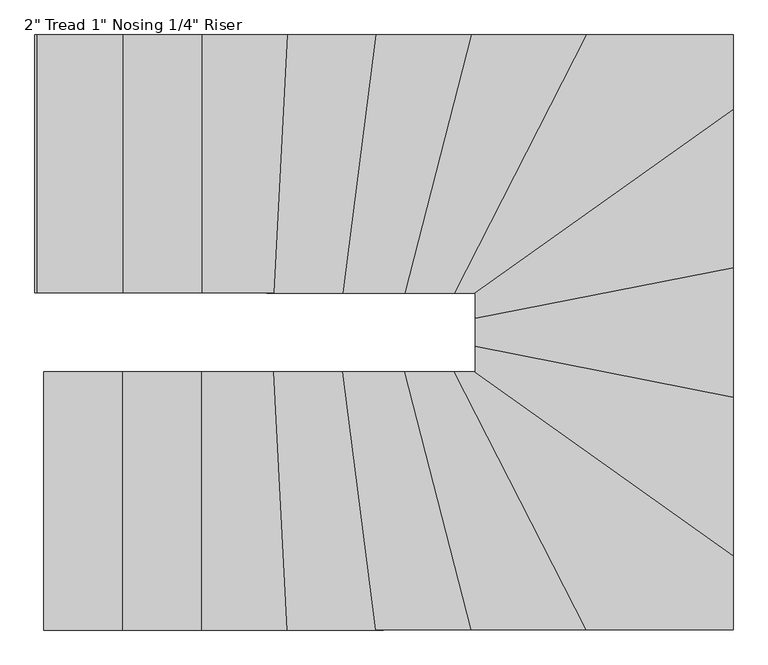
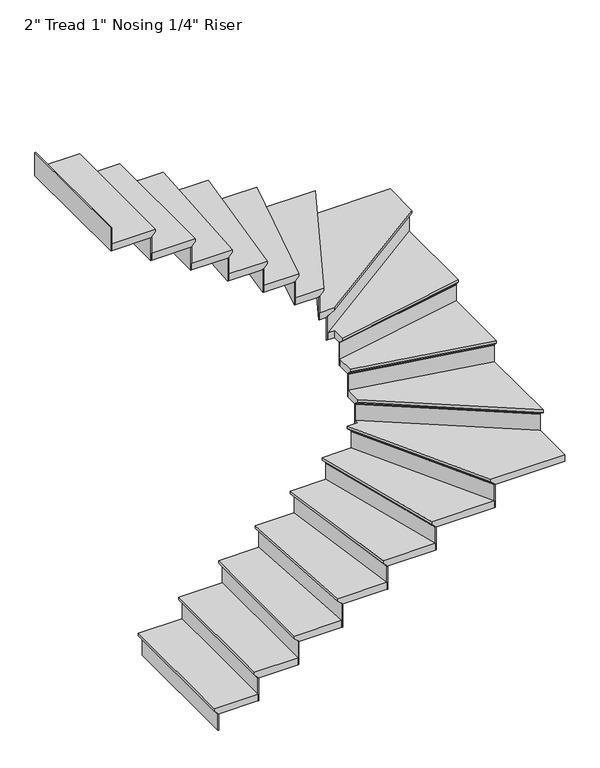
"""IFC4 building model written with IfcOpenShell, lengths in millimetres: stair flight geometry."""

from ifc_helpers import new_model, si_unit, origin, place, context, project, spatial, faceted_brep, source, transform, mapped, element, save


def stair_flight_4f848c3a(model_context):
    return source(origin(), model_context, "Body", "Brep", [
        faceted_brep([(531.7538115, -7565.2090409, 3350.6833333), (531.7538115, -7565.2090409, 3369.7333333), (531.7538115, -6650.8090409, 3369.7333333), (531.7538115, -6650.8090409, 3350.6833333), (557.1538115, -7565.2090409, 3325.2833333), (557.1538115, -6650.8090409, 3325.2833333), (836.5538115, -7565.2090409, 3369.7333333), (836.5538115, -6650.8090409, 3369.7333333), (557.1538115, -6650.8090409, 3318.9333333), (836.5538115, -6650.8090409, 3318.9333333), (836.5538115, -7565.2090409, 3318.9333333), (557.1538115, -7565.2090409, 3318.9333333)], [[[0, 1, 2, 3]], [[4, 0, 3, 5]], [[2, 1, 6, 7]], [[8, 9, 10, 11]], [[2, 7, 9, 8, 5, 3]], [[8, 11, 4, 5]], [[6, 1, 0, 4, 11, 10]], [[7, 6, 10, 9]]]),
        faceted_brep([(557.1538115, -7565.2090409, 3318.9333333), (557.1538115, -7565.2090409, 3200.4), (563.5038115, -7565.2090409, 3200.4), (563.5038115, -7565.2090409, 3318.9333333), (557.1538115, -6650.8090409, 3318.9333333), (563.5038115, -6650.8090409, 3318.9333333), (563.5038115, -6650.8090409, 3200.4), (557.1538115, -6650.8090409, 3200.4)], [[[0, 1, 2, 3]], [[4, 5, 6, 7]], [[1, 0, 4, 7]], [[2, 1, 7, 6]], [[3, 2, 6, 5]], [[0, 3, 5, 4]]]),
        faceted_brep([(836.5538115, -7565.2090409, 3488.2666667), (836.5538115, -7565.2090409, 3318.9333333), (842.9038115, -7565.2090409, 3318.9333333), (842.9038115, -7565.2090409, 3488.2666667), (836.5538115, -6650.8090409, 3488.2666667), (842.9038115, -6650.8090409, 3488.2666667), (842.9038115, -6650.8090409, 3318.9333333), (836.5538115, -6650.8090409, 3318.9333333)], [[[0, 1, 2, 3]], [[4, 5, 6, 7]], [[1, 0, 4, 7]], [[2, 1, 7, 6]], [[3, 2, 6, 5]], [[0, 3, 5, 4]]]),
        faceted_brep([(811.1538115, -6650.8090409, 3539.0666667), (811.1538115, -7565.2090409, 3539.0666667), (1115.9538115, -7565.2090409, 3539.0666667), (1115.9538115, -6650.8090409, 3539.0666667), (836.5538115, -6650.8090409, 3488.2666667), (1115.9538115, -6650.8090409, 3488.2666667), (1115.9538115, -7565.2090409, 3488.2666667), (836.5538115, -7565.2090409, 3488.2666667), (836.5538115, -6650.8090409, 3494.6166667), (811.1538115, -6650.8090409, 3520.0166667), (836.5538115, -7565.2090409, 3494.6166667), (811.1538115, -7565.2090409, 3520.0166667)], [[[0, 1, 2, 3]], [[4, 5, 6, 7]], [[0, 3, 5, 4, 8, 9]], [[4, 7, 10, 8]], [[2, 1, 11, 10, 7, 6]], [[3, 2, 6, 5]], [[11, 1, 0, 9]], [[10, 11, 9, 8]]]),
        faceted_brep([(1115.9538115, -7565.2090409, 3657.6), (1115.9538115, -7565.2090409, 3488.2666667), (1122.3038115, -7565.2090409, 3488.2666667), (1122.3038115, -7565.2090409, 3657.6), (1115.9538115, -6650.8090409, 3657.6), (1122.3038115, -6650.8090409, 3657.6), (1122.3038115, -6650.8090409, 3488.2666667), (1115.9538115, -6650.8090409, 3488.2666667)], [[[0, 1, 2, 3]], [[4, 5, 6, 7]], [[1, 0, 4, 7]], [[2, 1, 7, 6]], [[3, 2, 6, 5]], [[0, 3, 5, 4]]]),
        faceted_brep([(1090.5538115, -6650.8090409, 3708.4), (1090.5538115, -7565.2090409, 3708.4), (1419.1552434, -7565.2090409, 3708.4), (1371.620973, -6650.8090409, 3708.4), (1115.9538115, -6650.8090409, 3657.6), (1371.620973, -6650.8090409, 3657.6), (1419.1552434, -7565.2090409, 3657.6), (1115.9538115, -7565.2090409, 3657.6), (1115.9538115, -6650.8090409, 3663.95), (1090.5538115, -6650.8090409, 3689.35), (1115.9538115, -7565.2090409, 3663.95), (1090.5538115, -7565.2090409, 3689.35)], [[[0, 1, 2, 3]], [[4, 5, 6, 7]], [[0, 3, 5, 4, 8, 9]], [[4, 7, 10, 8]], [[2, 1, 11, 10, 7, 6]], [[3, 2, 6, 5]], [[11, 1, 0, 9]], [[10, 11, 9, 8]]]),
        faceted_brep([(1419.1552434, -7565.2090409, 3826.9333333), (1419.1552434, -7565.2090409, 3657.6), (1425.5138176, -7565.2090409, 3657.6), (1425.5138176, -7565.2090409, 3826.9333333), (1371.620973, -6650.8090409, 3826.9333333), (1377.9795471, -6650.8090409, 3826.9333333), (1377.9795471, -6650.8090409, 3657.6), (1371.620973, -6650.8090409, 3657.6)], [[[0, 1, 2, 3]], [[4, 5, 6, 7]], [[1, 0, 4, 7]], [[2, 1, 7, 6]], [[3, 2, 6, 5]], [[0, 3, 5, 4]]]),
        faceted_brep([(1346.1866763, -6650.8090409, 3877.7333333), (1393.7209467, -7565.2090409, 3877.7333333), (1734.1437245, -7565.2090409, 3877.7333333), (1615.7876728, -6650.8090409, 3877.7333333), (1371.620973, -6650.8090409, 3826.9333333), (1615.7876728, -6650.8090409, 3826.9333333), (1734.1437245, -7565.2090409, 3826.9333333), (1419.1552434, -7565.2090409, 3826.9333333), (1371.620973, -6650.8090409, 3833.2833333), (1346.1866763, -6650.8090409, 3858.6833333), (1419.1552434, -7565.2090409, 3833.2833333), (1393.7209467, -7565.2090409, 3858.6833333)], [[[0, 1, 2, 3]], [[4, 5, 6, 7]], [[0, 3, 5, 4, 8, 9]], [[4, 7, 10, 8]], [[2, 1, 11, 10, 7, 6]], [[3, 2, 6, 5]], [[11, 1, 0, 9]], [[10, 11, 9, 8]]]),
        faceted_brep([(1734.1437245, -7565.2090409, 3996.2666667), (1734.1437245, -7565.2090409, 3826.9333333), (1740.5466962, -7565.2090409, 3826.9333333), (1740.5466962, -7565.2090409, 3996.2666667), (1615.7876728, -6650.8090409, 3996.2666667), (1622.1906446, -6650.8090409, 3996.2666667), (1622.1906446, -6650.8090409, 3826.9333333), (1615.7876728, -6650.8090409, 3826.9333333)], [[[0, 1, 2, 3]], [[4, 5, 6, 7]], [[1, 0, 4, 7]], [[2, 1, 7, 6]], [[3, 2, 6, 5]], [[0, 3, 5, 4]]]),
        faceted_brep([(1590.1757857, -6650.8090409, 4047.0666667), (1708.5318374, -7565.2090409, 4047.0666667), (2072.5453427, -7565.2090409, 4047.0666667), (1837.4148953, -6650.8090409, 4047.0666667), (1615.7876728, -6650.8090409, 3996.2666667), (1837.4148953, -6650.8090409, 3996.2666667), (2072.5453427, -7565.2090409, 3996.2666667), (1734.1437245, -7565.2090409, 3996.2666667), (1615.7876728, -6650.8090409, 4002.6166667), (1590.1757857, -6650.8090409, 4028.0166667), (1734.1437245, -7565.2090409, 4002.6166667), (1708.5318374, -7565.2090409, 4028.0166667)], [[[0, 1, 2, 3]], [[4, 5, 6, 7]], [[0, 3, 5, 4, 8, 9]], [[4, 7, 10, 8]], [[2, 1, 11, 10, 7, 6]], [[3, 2, 6, 5]], [[11, 1, 0, 9]], [[10, 11, 9, 8]]]),
        faceted_brep([(2072.5453427, -7565.2090409, 4165.6), (2072.5453427, -7565.2090409, 3996.2666667), (2079.1019196, -7565.2090409, 3996.2666667), (2079.1019196, -7565.2090409, 4165.6), (1837.4148953, -6650.8090409, 4165.6), (1843.9714722, -6650.8090409, 4165.6), (1843.9714722, -6650.8090409, 3996.2666667), (1837.4148953, -6650.8090409, 3996.2666667)], [[[0, 1, 2, 3]], [[4, 5, 6, 7]], [[1, 0, 4, 7]], [[2, 1, 7, 6]], [[3, 2, 6, 5]], [[0, 3, 5, 4]]]),
        faceted_brep([(1811.1885878, -6650.8090409, 4216.4), (2046.3190352, -7565.2090409, 4216.4), (2482.5861527, -7565.2090409, 4216.4), (2013.7615314, -6650.8090409, 4216.4), (1837.4148953, -6650.8090409, 4165.6), (2013.7615314, -6650.8090409, 4165.6), (2482.5861527, -7565.2090409, 4165.6), (2072.5453427, -7565.2090409, 4165.6), (1837.4148953, -6650.8090409, 4171.95), (1811.1885878, -6650.8090409, 4197.35), (2072.5453427, -7565.2090409, 4171.95), (2046.3190352, -7565.2090409, 4197.35)], [[[0, 1, 2, 3]], [[4, 5, 6, 7]], [[0, 3, 5, 4, 8, 9]], [[4, 7, 10, 8]], [[2, 1, 11, 10, 7, 6]], [[3, 2, 6, 5]], [[11, 1, 0, 9]], [[10, 11, 9, 8]]]),
        faceted_brep([(2482.5861527, -7565.2090409, 4334.9333333), (2482.5861527, -7565.2090409, 4165.6), (2489.7221358, -7565.2090409, 4165.6), (2489.7221358, -7565.2090409, 4334.9333333), (2013.7615314, -6650.8090409, 4334.9333333), (2020.8975145, -6650.8090409, 4334.9333333), (2020.8975145, -6650.8090409, 4165.6), (2013.7615314, -6650.8090409, 4165.6)], [[[0, 1, 2, 3]], [[4, 5, 6, 7]], [[1, 0, 4, 7]], [[2, 1, 7, 6]], [[3, 2, 6, 5]], [[0, 3, 5, 4]]]),
        faceted_brep([(2059.4855034, -6621.253958, 4385.7333333), (2059.4855034, -6650.8090409, 4385.7333333), (1985.2175988, -6650.8090409, 4385.7333333), (2454.0422202, -7565.2090409, 4385.7333333), (2973.8855034, -7565.2090409, 4385.7333333), (2973.8855034, -7271.5279072, 4385.7333333), (2059.4855034, -6650.8090409, 4334.9333333), (2059.4855034, -6621.253958, 4334.9333333), (2973.8855034, -7271.5279072, 4334.9333333), (2973.8855034, -7565.2090409, 4334.9333333), (2482.5861527, -7565.2090409, 4334.9333333), (2013.7615314, -6650.8090409, 4334.9333333), (2013.7615314, -6650.8090409, 4341.2833333), (1985.2175988, -6650.8090409, 4366.6833333), (2482.5861527, -7565.2090409, 4341.2833333), (2454.0422202, -7565.2090409, 4366.6833333)], [[[0, 1, 2, 3, 4, 5]], [[6, 7, 8, 9, 10, 11]], [[1, 0, 7, 6]], [[2, 1, 6, 11, 12, 13]], [[11, 10, 14, 12]], [[4, 3, 15, 14, 10, 9]], [[5, 4, 9, 8]], [[0, 5, 8, 7]], [[15, 3, 2, 13]], [[14, 15, 13, 12]]]),
        faceted_brep([(2973.8855034, -7271.5279072, 4504.2666667), (2973.8855034, -7271.5279072, 4334.9333333), (2973.8855034, -7263.7359324, 4334.9333333), (2973.8855034, -7263.7359324, 4504.2666667), (2059.4855034, -6621.253958, 4504.2666667), (2059.4855034, -6613.4619832, 4504.2666667), (2059.4855034, -6613.4619832, 4334.9333333), (2059.4855034, -6621.253958, 4334.9333333)], [[[0, 1, 2, 3]], [[4, 5, 6, 7]], [[1, 0, 4, 7]], [[2, 1, 7, 6]], [[3, 2, 6, 5]], [[0, 3, 5, 4]]]),
        faceted_brep([(2059.4855034, -6652.4218572, 4555.0666667), (2973.8855034, -7302.6958063, 4555.0666667), (2973.8855034, -6715.0407273, 4555.0666667), (2059.4855034, -6534.7998709, 4555.0666667), (2059.4855034, -6621.253958, 4504.2666667), (2059.4855034, -6534.7998709, 4504.2666667), (2973.8855034, -6715.0407273, 4504.2666667), (2973.8855034, -7271.5279072, 4504.2666667), (2059.4855034, -6621.253958, 4510.6166667), (2059.4855034, -6652.4218572, 4536.0166667), (2973.8855034, -7271.5279072, 4510.6166667), (2973.8855034, -7302.6958063, 4536.0166667)], [[[0, 1, 2, 3]], [[4, 5, 6, 7]], [[0, 3, 5, 4, 8, 9]], [[4, 7, 10, 8]], [[3, 2, 6, 5]], [[11, 1, 0, 9]], [[10, 11, 9, 8]], [[2, 1, 11, 10, 7, 6]]]),
        faceted_brep([(2973.8855034, -6715.0407273, 4673.6), (2973.8855034, -6715.0407273, 4504.2666667), (2973.8855034, -6708.5685418, 4504.2666667), (2973.8855034, -6708.5685418, 4673.6), (2059.4855034, -6534.7998709, 4673.6), (2059.4855034, -6528.3276855, 4673.6), (2059.4855034, -6528.3276855, 4504.2666667), (2059.4855034, -6534.7998709, 4504.2666667)], [[[0, 1, 2, 3]], [[4, 5, 6, 7]], [[1, 0, 4, 7]], [[2, 1, 7, 6]], [[3, 2, 6, 5]], [[0, 3, 5, 4]]]),
        faceted_brep([(2059.4855034, -6560.6886127, 4724.4), (2973.8855034, -6740.929469, 4724.4), (2973.8855034, -6255.3998709, 4724.4), (2059.4855034, -6435.6407273, 4724.4), (2059.4855034, -6534.7998709, 4673.6), (2059.4855034, -6435.6407273, 4673.6), (2973.8855034, -6255.3998709, 4673.6), (2973.8855034, -6715.0407273, 4673.6), (2059.4855034, -6534.7998709, 4679.95), (2059.4855034, -6560.6886127, 4705.35), (2973.8855034, -6715.0407273, 4679.95), (2973.8855034, -6740.929469, 4705.35)], [[[0, 1, 2, 3]], [[4, 5, 6, 7]], [[0, 3, 5, 4, 8, 9]], [[4, 7, 10, 8]], [[2, 1, 11, 10, 7, 6]], [[3, 2, 6, 5]], [[11, 1, 0, 9]], [[10, 11, 9, 8]]]),
        faceted_brep([(2973.8855034, -6255.3998709, 4842.9333333), (2973.8855034, -6255.3998709, 4673.6), (2973.8855034, -6248.9276855, 4673.6), (2973.8855034, -6248.9276855, 4842.9333333), (2059.4855034, -6435.6407273, 4842.9333333), (2059.4855034, -6429.1685418, 4842.9333333), (2059.4855034, -6429.1685418, 4673.6), (2059.4855034, -6435.6407273, 4673.6)], [[[0, 1, 2, 3]], [[4, 5, 6, 7]], [[1, 0, 4, 7]], [[2, 1, 7, 6]], [[3, 2, 6, 5]], [[0, 3, 5, 4]]]),
        faceted_brep([(2013.3900289, -6371.4090409, 4893.7333333), (2059.4855034, -6371.4090409, 4893.7333333), (2059.4855034, -6461.529469, 4893.7333333), (2973.8855034, -6281.2886127, 4893.7333333), (2973.8855034, -5688.3543762, 4893.7333333), (2059.4855034, -6371.4090409, 4842.9333333), (2013.3900289, -6371.4090409, 4842.9333333), (2973.8855034, -5688.3543762, 4842.9333333), (2973.8855034, -6255.3998709, 4842.9333333), (2059.4855034, -6435.6407273, 4842.9333333), (2973.8855034, -6255.3998709, 4849.2833333), (2059.4855034, -6435.6407273, 4849.2833333), (2973.8855034, -6281.2886127, 4874.6833333), (2059.4855034, -6461.529469, 4874.6833333)], [[[0, 1, 2, 3, 4]], [[5, 6, 7, 8, 9]], [[1, 0, 6, 5]], [[9, 8, 10, 11]], [[4, 3, 12, 10, 8, 7]], [[0, 4, 7, 6]], [[12, 3, 2, 13]], [[10, 12, 13, 11]], [[2, 1, 5, 9, 11, 13]]]),
        faceted_brep([(2973.8855034, -5688.3543762, 5012.2666667), (2973.8855034, -5688.3543762, 4842.9333333), (2973.8855034, -5680.5624014, 4842.9333333), (2973.8855034, -5680.5624014, 5012.2666667), (2013.3900289, -6371.4090409, 5012.2666667), (2002.4331364, -6371.4090409, 5012.2666667), (2002.4331364, -6371.4090409, 4842.9333333), (2013.3900289, -6371.4090409, 4842.9333333)], [[[0, 1, 2, 3]], [[4, 5, 6, 7]], [[1, 0, 4, 7]], [[2, 1, 7, 6]], [[3, 2, 6, 5]], [[0, 3, 5, 4]]]),
        faceted_brep([(2057.2175988, -6371.4090409, 5063.0666667), (2973.8855034, -5719.5222754, 5063.0666667), (2973.8855034, -5457.0090409, 5063.0666667), (2425.4982876, -5457.0090409, 5063.0666667), (1956.6736663, -6371.4090409, 5063.0666667), (2013.3900289, -6371.4090409, 5012.2666667), (1956.6736663, -6371.4090409, 5012.2666667), (2425.4982876, -5457.0090409, 5012.2666667), (2973.8855034, -5457.0090409, 5012.2666667), (2973.8855034, -5688.3543762, 5012.2666667), (2013.3900289, -6371.4090409, 5018.6166667), (2057.2175988, -6371.4090409, 5044.0166667), (2973.8855034, -5688.3543762, 5018.6166667), (2973.8855034, -5719.5222754, 5044.0166667)], [[[0, 1, 2, 3, 4]], [[5, 6, 7, 8, 9]], [[0, 4, 6, 5, 10, 11]], [[5, 9, 12, 10]], [[2, 1, 13, 12, 9, 8]], [[4, 3, 7, 6]], [[13, 1, 0, 11]], [[12, 13, 11, 10]], [[3, 2, 8, 7]]]),
        faceted_brep([(2425.4982876, -5457.0090409, 5181.6), (2425.4982876, -5457.0090409, 5012.2666667), (2418.3623045, -5457.0090409, 5012.2666667), (2418.3623045, -5457.0090409, 5181.6), (1956.6736663, -6371.4090409, 5181.6), (1949.5376832, -6371.4090409, 5181.6), (1949.5376832, -6371.4090409, 5012.2666667), (1956.6736663, -6371.4090409, 5012.2666667)], [[[0, 1, 2, 3]], [[4, 5, 6, 7]], [[1, 0, 4, 7]], [[2, 1, 7, 6]], [[3, 2, 6, 5]], [[0, 3, 5, 4]]]),
        faceted_brep([(1985.2175988, -6371.4090409, 5232.4), (2454.0422202, -5457.0090409, 5232.4), (2020.0927278, -5457.0090409, 5232.4), (1784.9622804, -6371.4090409, 5232.4), (1956.6736663, -6371.4090409, 5181.6), (1784.9622804, -6371.4090409, 5181.6), (2020.0927278, -5457.0090409, 5181.6), (2425.4982876, -5457.0090409, 5181.6), (1956.6736663, -6371.4090409, 5187.95), (1985.2175988, -6371.4090409, 5213.35), (2425.4982876, -5457.0090409, 5187.95), (2454.0422202, -5457.0090409, 5213.35)], [[[0, 1, 2, 3]], [[4, 5, 6, 7]], [[0, 3, 5, 4, 8, 9]], [[4, 7, 10, 8]], [[2, 1, 11, 10, 7, 6]], [[3, 2, 6, 5]], [[11, 1, 0, 9]], [[10, 11, 9, 8]]]),
        faceted_brep([(2020.0927278, -5457.0090409, 5350.9333333), (2020.0927278, -5457.0090409, 5181.6), (2013.5361509, -5457.0090409, 5181.6), (2013.5361509, -5457.0090409, 5350.9333333), (1784.9622804, -6371.4090409, 5350.9333333), (1778.4057035, -6371.4090409, 5350.9333333), (1778.4057035, -6371.4090409, 5181.6), (1784.9622804, -6371.4090409, 5181.6)], [[[0, 1, 2, 3]], [[4, 5, 6, 7]], [[1, 0, 4, 7]], [[2, 1, 7, 6]], [[3, 2, 6, 5]], [[0, 3, 5, 4]]]),
        faceted_brep([(1811.1885878, -6371.4090409, 5401.7333333), (2046.3190352, -5457.0090409, 5401.7333333), (1682.9199502, -5457.0090409, 5401.7333333), (1564.5638986, -6371.4090409, 5401.7333333), (1784.9622804, -6371.4090409, 5350.9333333), (1564.5638986, -6371.4090409, 5350.9333333), (1682.9199502, -5457.0090409, 5350.9333333), (2020.0927278, -5457.0090409, 5350.9333333), (1784.9622804, -6371.4090409, 5357.2833333), (1811.1885878, -6371.4090409, 5382.6833333), (2020.0927278, -5457.0090409, 5357.2833333), (2046.3190352, -5457.0090409, 5382.6833333)], [[[0, 1, 2, 3]], [[4, 5, 6, 7]], [[0, 3, 5, 4, 8, 9]], [[4, 7, 10, 8]], [[2, 1, 11, 10, 7, 6]], [[3, 2, 6, 5]], [[11, 1, 0, 9]], [[10, 11, 9, 8]]]),
        faceted_brep([(1682.9199502, -5457.0090409, 5520.2666667), (1682.9199502, -5457.0090409, 5350.9333333), (1676.5169785, -5457.0090409, 5350.9333333), (1676.5169785, -5457.0090409, 5520.2666667), (1564.5638986, -6371.4090409, 5520.2666667), (1558.1609268, -6371.4090409, 5520.2666667), (1558.1609268, -6371.4090409, 5350.9333333), (1564.5638986, -6371.4090409, 5350.9333333)], [[[0, 1, 2, 3]], [[4, 5, 6, 7]], [[1, 0, 4, 7]], [[2, 1, 7, 6]], [[3, 2, 6, 5]], [[0, 3, 5, 4]]]),
        faceted_brep([(1590.1757857, -6371.4090409, 5571.0666667), (1708.5318374, -5457.0090409, 5571.0666667), (1368.2866501, -5457.0090409, 5571.0666667), (1320.7523797, -6371.4090409, 5571.0666667), (1564.5638986, -6371.4090409, 5520.2666667), (1320.7523797, -6371.4090409, 5520.2666667), (1368.2866501, -5457.0090409, 5520.2666667), (1682.9199502, -5457.0090409, 5520.2666667), (1564.5638986, -6371.4090409, 5526.6166667), (1590.1757857, -6371.4090409, 5552.0166667), (1682.9199502, -5457.0090409, 5526.6166667), (1708.5318374, -5457.0090409, 5552.0166667)], [[[0, 1, 2, 3]], [[4, 5, 6, 7]], [[0, 3, 5, 4, 8, 9]], [[4, 7, 10, 8]], [[2, 1, 11, 10, 7, 6]], [[3, 2, 6, 5]], [[11, 1, 0, 9]], [[10, 11, 9, 8]]]),
        faceted_brep([(1368.2866501, -5457.0090409, 5689.6), (1368.2866501, -5457.0090409, 5520.2666667), (1361.9280759, -5457.0090409, 5520.2666667), (1361.9280759, -5457.0090409, 5689.6), (1320.7523797, -6371.4090409, 5689.6), (1314.3938055, -6371.4090409, 5689.6), (1314.3938055, -6371.4090409, 5520.2666667), (1320.7523797, -6371.4090409, 5520.2666667)], [[[0, 1, 2, 3]], [[4, 5, 6, 7]], [[1, 0, 4, 7]], [[2, 1, 7, 6]], [[3, 2, 6, 5]], [[0, 3, 5, 4]]]),
        faceted_brep([(1346.1866763, -6371.4090409, 5740.4), (1393.7209467, -5457.0090409, 5740.4), (1065.1538115, -5457.0090409, 5740.4), (1065.1538115, -6371.4090409, 5740.4), (1320.7523797, -6371.4090409, 5689.6), (1065.1538115, -6371.4090409, 5689.6), (1065.1538115, -5457.0090409, 5689.6), (1368.2866501, -5457.0090409, 5689.6), (1320.7523797, -6371.4090409, 5695.95), (1346.1866763, -6371.4090409, 5721.35), (1368.2866501, -5457.0090409, 5695.95), (1393.7209467, -5457.0090409, 5721.35)], [[[0, 1, 2, 3]], [[4, 5, 6, 7]], [[0, 3, 5, 4, 8, 9]], [[4, 7, 10, 8]], [[2, 1, 11, 10, 7, 6]], [[3, 2, 6, 5]], [[11, 1, 0, 9]], [[10, 11, 9, 8]]]),
        faceted_brep([(1065.1538115, -5457.0090409, 5858.9333333), (1065.1538115, -5457.0090409, 5689.6), (1058.8038115, -5457.0090409, 5689.6), (1058.8038115, -5457.0090409, 5858.9333333), (1065.1538115, -6371.4090409, 5858.9333333), (1058.8038115, -6371.4090409, 5858.9333333), (1058.8038115, -6371.4090409, 5689.6), (1065.1538115, -6371.4090409, 5689.6)], [[[0, 1, 2, 3]], [[4, 5, 6, 7]], [[1, 0, 4, 7]], [[2, 1, 7, 6]], [[3, 2, 6, 5]], [[0, 3, 5, 4]]]),
        faceted_brep([(1090.5538115, -6371.4090409, 5909.7333333), (1090.5538115, -5457.0090409, 5909.7333333), (785.7538115, -5457.0090409, 5909.7333333), (785.7538115, -6371.4090409, 5909.7333333), (1065.1538115, -6371.4090409, 5858.9333333), (785.7538115, -6371.4090409, 5858.9333333), (785.7538115, -5457.0090409, 5858.9333333), (1065.1538115, -5457.0090409, 5858.9333333), (1065.1538115, -6371.4090409, 5865.2833333), (1090.5538115, -6371.4090409, 5890.6833333), (1065.1538115, -5457.0090409, 5865.2833333), (1090.5538115, -5457.0090409, 5890.6833333)], [[[0, 1, 2, 3]], [[4, 5, 6, 7]], [[0, 3, 5, 4, 8, 9]], [[4, 7, 10, 8]], [[2, 1, 11, 10, 7, 6]], [[3, 2, 6, 5]], [[11, 1, 0, 9]], [[10, 11, 9, 8]]]),
        faceted_brep([(785.7538115, -5457.0090409, 6028.2666667), (785.7538115, -5457.0090409, 5858.9333333), (779.4038115, -5457.0090409, 5858.9333333), (779.4038115, -5457.0090409, 6028.2666667), (785.7538115, -6371.4090409, 6028.2666667), (779.4038115, -6371.4090409, 6028.2666667), (779.4038115, -6371.4090409, 5858.9333333), (785.7538115, -6371.4090409, 5858.9333333)], [[[0, 1, 2, 3]], [[4, 5, 6, 7]], [[1, 0, 4, 7]], [[2, 1, 7, 6]], [[3, 2, 6, 5]], [[0, 3, 5, 4]]]),
        faceted_brep([(506.3538115, -5457.0090409, 6197.6), (506.3538115, -5457.0090409, 6028.2666667), (500.0038115, -5457.0090409, 6028.2666667), (500.0038115, -5457.0090409, 6197.6), (506.3538115, -6371.4090409, 6197.6), (500.0038115, -6371.4090409, 6197.6), (500.0038115, -6371.4090409, 6028.2666667), (506.3538115, -6371.4090409, 6028.2666667)], [[[0, 1, 2, 3]], [[4, 5, 6, 7]], [[1, 0, 4, 7]], [[2, 1, 7, 6]], [[3, 2, 6, 5]], [[0, 3, 5, 4]]]),
        faceted_brep([(811.1538115, -6371.4090409, 6079.0666667), (811.1538115, -5457.0090409, 6079.0666667), (506.3538115, -5457.0090409, 6079.0666667), (506.3538115, -6371.4090409, 6079.0666667), (785.7538115, -6371.4090409, 6028.2666667), (506.3538115, -6371.4090409, 6028.2666667), (506.3538115, -5457.0090409, 6028.2666667), (785.7538115, -5457.0090409, 6028.2666667), (785.7538115, -6371.4090409, 6034.6166667), (811.1538115, -6371.4090409, 6060.0166667), (785.7538115, -5457.0090409, 6034.6166667), (811.1538115, -5457.0090409, 6060.0166667)], [[[0, 1, 2, 3]], [[4, 5, 6, 7]], [[0, 3, 5, 4, 8, 9]], [[4, 7, 10, 8]], [[2, 1, 11, 10, 7, 6]], [[3, 2, 6, 5]], [[11, 1, 0, 9]], [[10, 11, 9, 8]]]),
    ])


if __name__ == "__main__":
    model = new_model("IFC4")
    model_context = context("Model", 3, world=origin())
    ifc_project = project(units=[si_unit("LENGTHUNIT", "METRE", prefix="MILLI")], contexts=[model_context])
    site = spatial("IfcSite", under=ifc_project)
    building = spatial("IfcBuilding", under=site)
    placement = place(None, origin())
    stair_flight_shape = stair_flight_4f848c3a(model_context)
    element("IfcStairFlight", 1, ObjectType="2\" Tread 1\" Nosing 1/4\" Riser", at=placement, inside=building, context=model_context, shape_type="MappedRepresentation", body=[
        mapped(stair_flight_shape, transform((0.0, 0.0, 0.0), x_axis=(1.0, 0.0, 0.0), y_axis=(0.0, 1.0, 0.0), z_axis=(0.0, 0.0, 1.0))),
    ])
    save(model, "model.ifc")
